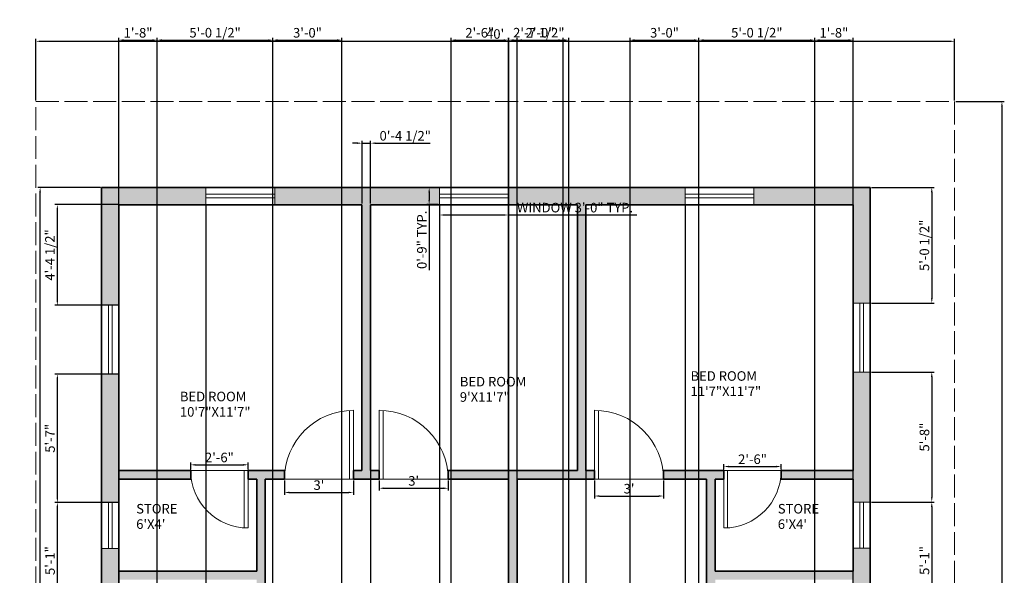
# Model space of a CAD drawing. Units: inches. Extents: x 2871 to 3419, y 1549 to 2228.
# Tile 3 of 3: x 2905 to 3419, y 1938 to 2228. Entities that reach past the tile are written whole.
import ezdxf

# ---------------------------------------------------------------- set-up
doc = ezdxf.new("R2010")
doc.units = ezdxf.units.IN
doc.linetypes.add('ACAD_ISO02W100', pattern=[15, 12, -3])
for name, color, linetype, lineweight in [('A-ANNO-DIMS', 3, 'Continuous', 13), ('A-AREA-IDEN', 3, 'Continuous', 18), ('A-WALL-PATT', 18, 'Continuous', 13), ('C-PROP', 7, 'ACAD_ISO02W100', 18), ('doors', 6, 'Continuous', 18), ('wall', 4, 'Continuous', 35), ('windows', 1, 'Continuous', 18)]:
    doc.layers.add(name, color=color, linetype=linetype, lineweight=lineweight)
doc.styles.get("Standard").update_dxf_attribs({"font": 'arial.ttf', "height": 5})
doc.dimstyles.new('ISO-25', dxfattribs={"dimtxt": 5, "dimasz": 2.5, "dimexe": 1.25, "dimexo": 0.625, "dimtad": 1, "dimlunit": 3, "dimtxsty": 'Standard', "dimcen": 2.5, "dimadec": 0, "dimazin": 0, "dimtfac": 1, "dimtmove": 0, "dimatfit": 3, "dimfxl": 1, "dimarcsym": 0})

# ---------------------------------------------------------------- blocks, each defined once
blk = doc.blocks.new('*D1')
at = {"layer": 'A-ANNO-DIMS', "color": 0, "lineweight": -2, "transparency": 16777216}
for p, q in [((3092.92, 1987.61), (3092.92, 1982.26)), ((3128.92, 1987.61), (3128.92, 1982.26)), ((3095.42, 1983.51), (3126.42, 1983.51))]:
    blk.add_line(p, q, dxfattribs=at)
at = {"layer": 'A-ANNO-DIMS', "color": 0, "transparency": 16777216}
for points in [[(3095.42, 1983.92), (3095.42, 1983.09), (3092.92, 1983.51)], [(3126.42, 1983.92), (3126.42, 1983.09), (3128.92, 1983.51)]]:
    blk.add_solid(points, dxfattribs=at)
at = {"layer": 'Defpoints', "color": 0, "transparency": 16777216}
for p in [(3092.92, 1988.24), (3128.92, 1988.24), (3128.92, 1983.51)]:
    blk.add_point(p, dxfattribs=at)
at = {"layer": 'A-ANNO-DIMS', "color": 0, "transparency": 16777216, "insert": (3110.92, 1986.69), "char_height": 5, "attachment_point": 5}
blk.add_mtext("3'", dxfattribs=at)
blk = doc.blocks.new('*D2')
at = {"layer": 'A-ANNO-DIMS', "color": 0, "lineweight": -2, "transparency": 16777216}
for p, q in [((3043.42, 1987.61), (3043.42, 1980.06)), ((3079.42, 1987.61), (3079.42, 1980.06)), ((3045.92, 1981.31), (3076.92, 1981.31))]:
    blk.add_line(p, q, dxfattribs=at)
at = {"layer": 'A-ANNO-DIMS', "color": 0, "transparency": 16777216}
for points in [[(3045.92, 1981.72), (3045.92, 1980.89), (3043.42, 1981.31)], [(3076.92, 1981.72), (3076.92, 1980.89), (3079.42, 1981.31)]]:
    blk.add_solid(points, dxfattribs=at)
at = {"layer": 'Defpoints', "color": 0, "transparency": 16777216}
for p in [(3043.42, 1988.24), (3079.42, 1988.24), (3079.42, 1981.31)]:
    blk.add_point(p, dxfattribs=at)
at = {"layer": 'A-ANNO-DIMS', "color": 0, "transparency": 16777216, "insert": (3061.42, 1984.49), "char_height": 5, "attachment_point": 5}
blk.add_mtext("3'", dxfattribs=at)
blk = doc.blocks.new('*D3')
at = {"layer": 'A-ANNO-DIMS', "color": 0, "lineweight": -2, "transparency": 16777216}
for p, q in [((2994.42, 1993.36), (2994.42, 1997)), ((2996.92, 1995.75), (3021.92, 1995.75)), ((3024.42, 1993.36), (3024.42, 1997))]:
    blk.add_line(p, q, dxfattribs=at)
at = {"layer": 'A-ANNO-DIMS', "color": 0, "transparency": 16777216}
for points in [[(2996.92, 1996.17), (2996.92, 1995.33), (2994.42, 1995.75)], [(3021.92, 1996.17), (3021.92, 1995.33), (3024.42, 1995.75)]]:
    blk.add_solid(points, dxfattribs=at)
at = {"layer": 'Defpoints', "color": 0, "transparency": 16777216}
for p in [(3024.42, 1995.75), (2994.42, 1992.74), (3024.42, 1992.74)]:
    blk.add_point(p, dxfattribs=at)
at = {"layer": 'A-ANNO-DIMS', "color": 0, "transparency": 16777216, "insert": (3009.42, 1998.93), "char_height": 5, "attachment_point": 5}
blk.add_mtext('2\'-6"', dxfattribs=at)
blk = doc.blocks.new('*D4')
at = {"layer": 'A-ANNO-DIMS', "color": 0, "lineweight": -2, "transparency": 16777216}
for p, q in [((3205.42, 1987.61), (3205.42, 1978.19)), ((3241.42, 1987.61), (3241.42, 1978.19)), ((3207.92, 1979.44), (3238.92, 1979.44))]:
    blk.add_line(p, q, dxfattribs=at)
at = {"layer": 'A-ANNO-DIMS', "color": 0, "transparency": 16777216}
for points in [[(3207.92, 1979.86), (3207.92, 1979.02), (3205.42, 1979.44)], [(3238.92, 1979.86), (3238.92, 1979.02), (3241.42, 1979.44)]]:
    blk.add_solid(points, dxfattribs=at)
at = {"layer": 'Defpoints', "color": 0, "transparency": 16777216}
for p in [(3205.42, 1988.24), (3241.42, 1988.24), (3241.42, 1979.44)]:
    blk.add_point(p, dxfattribs=at)
at = {"layer": 'A-ANNO-DIMS', "color": 0, "transparency": 16777216, "insert": (3223.42, 1982.62), "char_height": 5, "attachment_point": 5}
blk.add_mtext("3'", dxfattribs=at)
blk = doc.blocks.new('*D5')
at = {"layer": 'A-ANNO-DIMS', "color": 0, "lineweight": -2, "transparency": 16777216}
for p, q in [((3272.92, 1993.36), (3272.92, 1996.1)), ((3302.92, 1993.36), (3302.92, 1996.1)), ((3275.42, 1994.85), (3300.42, 1994.85))]:
    blk.add_line(p, q, dxfattribs=at)
at = {"layer": 'A-ANNO-DIMS', "color": 0, "transparency": 16777216}
for points in [[(3275.42, 1995.27), (3275.42, 1994.43), (3272.92, 1994.85)], [(3300.42, 1995.27), (3300.42, 1994.43), (3302.92, 1994.85)]]:
    blk.add_solid(points, dxfattribs=at)
at = {"layer": 'Defpoints', "color": 0, "transparency": 16777216}
for p in [(3272.92, 1992.74), (3302.92, 1994.85), (3302.92, 1992.74)]:
    blk.add_point(p, dxfattribs=at)
at = {"layer": 'A-ANNO-DIMS', "color": 0, "transparency": 16777216, "insert": (3287.92, 1998.03), "char_height": 5, "attachment_point": 5}
blk.add_mtext('2\'-6"', dxfattribs=at)
blk = doc.blocks.new('*D12')
at = {"layer": 'A-ANNO-DIMS', "color": 0, "lineweight": -2, "transparency": 16777216}
for p, q in [((2913.47, 2186.25), (2913.47, 2218.38)), ((2915.97, 2217.13), (3390.97, 2217.13)), ((3393.47, 2186.25), (3393.47, 2218.38))]:
    blk.add_line(p, q, dxfattribs=at)
at = {"layer": 'A-ANNO-DIMS', "color": 0, "transparency": 16777216}
for points in [[(2915.97, 2217.55), (2915.97, 2216.72), (2913.47, 2217.13)], [(3390.97, 2217.55), (3390.97, 2216.72), (3393.47, 2217.13)]]:
    blk.add_solid(points, dxfattribs=at)
at = {"layer": 'Defpoints', "color": 0, "transparency": 16777216}
for p in [(3393.47, 2217.13), (2913.47, 2185.62), (3393.47, 2185.62)]:
    blk.add_point(p, dxfattribs=at)
at = {"layer": 'A-ANNO-DIMS', "color": 0, "transparency": 16777216, "insert": (3153.47, 2220.31), "char_height": 5, "attachment_point": 5}
blk.add_mtext("40'", dxfattribs=at)
blk = doc.blocks.new('*D13')
at = {"layer": 'A-ANNO-DIMS', "color": 0, "lineweight": -2, "transparency": 16777216}
for p, q in [((3394.09, 2185.62), (3419.45, 2185.62)), ((3418.2, 2183.12), (3418.2, 1588.12)), ((3394.09, 1585.62), (3419.45, 1585.62))]:
    blk.add_line(p, q, dxfattribs=at)
at = {"layer": 'A-ANNO-DIMS', "color": 0, "transparency": 16777216}
for points in [[(3417.79, 2183.12), (3418.62, 2183.12), (3418.2, 2185.62)], [(3417.79, 1588.12), (3418.62, 1588.12), (3418.2, 1585.62)]]:
    blk.add_solid(points, dxfattribs=at)
at = {"layer": 'Defpoints', "color": 0, "transparency": 16777216}
for p in [(3393.47, 2185.62), (3393.47, 1585.62), (3418.2, 1585.62)]:
    blk.add_point(p, dxfattribs=at)
at = {"layer": 'A-ANNO-DIMS', "color": 0, "transparency": 16777216, "insert": (3415.03, 1885.62), "char_height": 5, "attachment_point": 5, "rotation": 90}
blk.add_mtext("50'", dxfattribs=at)
blk = doc.blocks.new('WIN-36IN')
for p, q in [((0, 36), (0, 0)), ((9, 36), (0, 36)), ((3.5, 0), (3.5, 36)), ((5.5, 0), (5.5, 36)), ((9, 0), (9, 36)), ((0, 0), (9, 0))]:
    blk.add_line(p, q)
blk = doc.blocks.new('WIN-24IN')
for p, q in [((0, 24), (0, 0)), ((9, 24), (0, 24)), ((3.5, 0), (3.5, 24)), ((5.5, 0), (5.5, 24)), ((9, 0), (9, 24)), ((0, 0), (9, 0))]:
    blk.add_line(p, q)
blk = doc.blocks.new('DOOR-SWING-30IN')
for p, q in [((28, 29.93), (28, 0)), ((30, 30), (30, 0)), ((30, 0), (0, 0))]:
    blk.add_line(p, q)
blk.add_arc((30, 0), 30, 90, 180)
blk = doc.blocks.new('DOOR-SWING-36IN')
for p, q in [((0, 36), (0, 0)), ((2, 35.94), (2, 0)), ((0, 0), (36, 0))]:
    blk.add_line(p, q)
blk.add_arc((0, 0), 36, 0, 90)
blk = doc.blocks.new('*D18')
at = {"layer": 'A-ANNO-DIMS', "color": 0, "lineweight": -2, "transparency": 16777216}
for p, q in [((3124.42, 2131.11), (3124.42, 2125.09)), ((3160.42, 2131.11), (3160.42, 2125.09)), ((3126.92, 2126.34), (3157.92, 2126.34)), ((3160.42, 2126.34), (3227.44, 2126.34))]:
    blk.add_line(p, q, dxfattribs=at)
at = {"layer": 'A-ANNO-DIMS', "color": 0, "transparency": 16777216}
for points in [[(3126.92, 2126.75), (3126.92, 2125.92), (3124.42, 2126.34)], [(3157.92, 2126.75), (3157.92, 2125.92), (3160.42, 2126.34)]]:
    blk.add_solid(points, dxfattribs=at)
at = {"layer": 'Defpoints', "color": 0, "transparency": 16777216}
for p in [(3124.42, 2131.74), (3160.42, 2131.74), (3160.42, 2126.34)]:
    blk.add_point(p, dxfattribs=at)
at = {"layer": 'A-ANNO-DIMS', "color": 0, "transparency": 16777216, "insert": (3195.18, 2129.55), "char_height": 5, "attachment_point": 5}
blk.add_mtext('WINDOW 3\'-0" TYP.', dxfattribs=at)
blk = doc.blocks.new('*D19')
at = {"layer": 'A-ANNO-DIMS', "color": 0, "lineweight": -2, "transparency": 16777216}
for p, q in [((3123.79, 2140.74), (3117.77, 2140.74)), ((3119.02, 2138.24), (3119.02, 2134.24)), ((3123.79, 2131.74), (3117.77, 2131.74)), ((3119.02, 2131.74), (3119.02, 2097.51))]:
    blk.add_line(p, q, dxfattribs=at)
at = {"layer": 'A-ANNO-DIMS', "color": 0, "transparency": 16777216}
for points in [[(3118.6, 2138.24), (3119.43, 2138.24), (3119.02, 2140.74)], [(3118.6, 2134.24), (3119.43, 2134.24), (3119.02, 2131.74)]]:
    blk.add_solid(points, dxfattribs=at)
at = {"layer": 'Defpoints', "color": 0, "transparency": 16777216}
for p in [(3124.42, 2140.74), (3119.02, 2131.74), (3124.42, 2131.74)]:
    blk.add_point(p, dxfattribs=at)
at = {"layer": 'A-ANNO-DIMS', "color": 0, "transparency": 16777216, "insert": (3115.84, 2113.37), "char_height": 5, "attachment_point": 5, "rotation": 90}
blk.add_mtext('0\'-9" TYP.', dxfattribs=at)
blk = doc.blocks.new('*D23')
at = {"layer": 'A-ANNO-DIMS', "color": 0, "lineweight": -2, "transparency": 16777216}
for p, q in [((2947.29, 2140.74), (2914.52, 2140.74)), ((2915.77, 1635.74), (2915.77, 2138.24)), ((2947.29, 1633.24), (2914.52, 1633.24))]:
    blk.add_line(p, q, dxfattribs=at)
at = {"layer": 'A-ANNO-DIMS', "color": 0, "transparency": 16777216}
for points in [[(2915.35, 2138.24), (2916.18, 2138.24), (2915.77, 2140.74)], [(2915.35, 1635.74), (2916.18, 1635.74), (2915.77, 1633.24)]]:
    blk.add_solid(points, dxfattribs=at)
at = {"layer": 'Defpoints', "color": 0, "transparency": 16777216}
for p in [(2915.77, 2140.74), (2947.92, 2140.74), (2947.92, 1633.24)]:
    blk.add_point(p, dxfattribs=at)
at = {"layer": 'A-ANNO-DIMS', "color": 0, "transparency": 16777216, "insert": (2912.56, 1886.99), "char_height": 5, "attachment_point": 5, "rotation": 90}
blk.add_mtext('42\'-3 1/2"', dxfattribs=at)
blk = doc.blocks.new('*D26')
at = {"layer": 'A-ANNO-DIMS', "color": 0, "lineweight": -2, "transparency": 16777216}
for p, q in [((2956.92, 2131.11), (2956.92, 1552.22)), ((3002.42, 2131.11), (3002.42, 1552.22)), ((2959.42, 1553.47), (2999.92, 1553.47))]:
    blk.add_line(p, q, dxfattribs=at)
at = {"layer": 'A-ANNO-DIMS', "color": 0, "transparency": 16777216}
for points in [[(2959.42, 1553.89), (2959.42, 1553.05), (2956.92, 1553.47)], [(2999.92, 1553.89), (2999.92, 1553.05), (3002.42, 1553.47)]]:
    blk.add_solid(points, dxfattribs=at)
at = {"layer": 'Defpoints', "color": 0, "transparency": 16777216}
for p in [(2956.92, 2131.74), (3002.42, 2131.74), (3002.42, 1553.47)]:
    blk.add_point(p, dxfattribs=at)
at = {"layer": 'A-ANNO-DIMS', "color": 0, "transparency": 16777216, "insert": (2979.67, 1556.68), "char_height": 5, "attachment_point": 5}
blk.add_mtext('3\'-9 1/2"', dxfattribs=at)
blk = doc.blocks.new('*D27')
at = {"layer": 'A-ANNO-DIMS', "color": 0, "lineweight": -2, "transparency": 16777216}
for p, q in [((3088.42, 2131.11), (3088.42, 1552.22)), ((3124.42, 2131.11), (3124.42, 1552.22)), ((3090.92, 1553.47), (3121.92, 1553.47))]:
    blk.add_line(p, q, dxfattribs=at)
at = {"layer": 'A-ANNO-DIMS', "color": 0, "transparency": 16777216}
for points in [[(3090.92, 1553.89), (3090.92, 1553.05), (3088.42, 1553.47)], [(3121.92, 1553.89), (3121.92, 1553.05), (3124.42, 1553.47)]]:
    blk.add_solid(points, dxfattribs=at)
at = {"layer": 'Defpoints', "color": 0, "transparency": 16777216}
for p in [(3088.42, 2131.74), (3124.42, 2131.74), (3124.42, 1553.47)]:
    blk.add_point(p, dxfattribs=at)
at = {"layer": 'A-ANNO-DIMS', "color": 0, "transparency": 16777216, "insert": (3106.42, 1556.65), "char_height": 5, "attachment_point": 5}
blk.add_mtext('3\'-0"', dxfattribs=at)
blk = doc.blocks.new('*D28')
at = {"layer": 'A-ANNO-DIMS', "color": 0, "lineweight": -2, "transparency": 16777216}
for p, q in [((3200.92, 2131.11), (3200.92, 1552.22)), ((3252.67, 2131.11), (3252.67, 1552.22)), ((3203.42, 1553.47), (3250.17, 1553.47))]:
    blk.add_line(p, q, dxfattribs=at)
at = {"layer": 'A-ANNO-DIMS', "color": 0, "transparency": 16777216}
for points in [[(3203.42, 1553.89), (3203.42, 1553.05), (3200.92, 1553.47)], [(3250.17, 1553.89), (3250.17, 1553.05), (3252.67, 1553.47)]]:
    blk.add_solid(points, dxfattribs=at)
at = {"layer": 'Defpoints', "color": 0, "transparency": 16777216}
for p in [(3200.92, 2131.74), (3252.67, 2131.74), (3252.67, 1553.47)]:
    blk.add_point(p, dxfattribs=at)
at = {"layer": 'A-ANNO-DIMS', "color": 0, "transparency": 16777216, "insert": (3226.79, 1556.6), "char_height": 5, "attachment_point": 5}
blk.add_mtext('4\'-4"', dxfattribs=at)
blk = doc.blocks.new('*D29')
at = {"layer": 'A-ANNO-DIMS', "color": 0, "lineweight": -2, "transparency": 16777216}
for p, q in [((3130.42, 1871.36), (3130.42, 2219.02)), ((3132.92, 2217.77), (3157.92, 2217.77)), ((3160.42, 1871.36), (3160.42, 2219.02))]:
    blk.add_line(p, q, dxfattribs=at)
at = {"layer": 'A-ANNO-DIMS', "color": 0, "transparency": 16777216}
for points in [[(3132.92, 2218.19), (3132.92, 2217.35), (3130.42, 2217.77)], [(3157.92, 2218.19), (3157.92, 2217.35), (3160.42, 2217.77)]]:
    blk.add_solid(points, dxfattribs=at)
at = {"layer": 'Defpoints', "color": 0, "transparency": 16777216}
for p in [(3160.42, 2217.77), (3130.42, 1870.74), (3160.42, 1870.74)]:
    blk.add_point(p, dxfattribs=at)
at = {"layer": 'A-ANNO-DIMS', "color": 0, "transparency": 16777216, "insert": (3145.42, 2220.95), "char_height": 5, "attachment_point": 5}
blk.add_mtext('2\'-6"', dxfattribs=at)
blk = doc.blocks.new('*D30')
at = {"layer": 'A-ANNO-DIMS', "color": 0, "lineweight": -2, "transparency": 16777216}
for p, q in [((3164.92, 1871.36), (3164.92, 2219.02)), ((3167.42, 2217.77), (3186.42, 2217.77)), ((3188.92, 1871.36), (3188.92, 2219.02))]:
    blk.add_line(p, q, dxfattribs=at)
at = {"layer": 'A-ANNO-DIMS', "color": 0, "transparency": 16777216}
for points in [[(3167.42, 2218.19), (3167.42, 2217.35), (3164.92, 2217.77)], [(3186.42, 2218.19), (3186.42, 2217.35), (3188.92, 2217.77)]]:
    blk.add_solid(points, dxfattribs=at)
at = {"layer": 'Defpoints', "color": 0, "transparency": 16777216}
for p in [(3188.92, 2217.77), (3164.92, 1870.74), (3188.92, 1870.74)]:
    blk.add_point(p, dxfattribs=at)
at = {"layer": 'A-ANNO-DIMS', "color": 0, "transparency": 16777216, "insert": (3176.92, 2220.95), "char_height": 5, "attachment_point": 5}
blk.add_mtext('2\'-0"', dxfattribs=at)
blk = doc.blocks.new('*D34')
at = {"layer": 'A-ANNO-DIMS', "color": 0, "lineweight": -2, "transparency": 16777216}
for p, q in [((3350.04, 2140.74), (3382.82, 2140.74)), ((3381.57, 2138.24), (3381.57, 2082.74)), ((3350.04, 2080.24), (3382.82, 2080.24))]:
    blk.add_line(p, q, dxfattribs=at)
at = {"layer": 'A-ANNO-DIMS', "color": 0, "transparency": 16777216}
for points in [[(3381.15, 2138.24), (3381.98, 2138.24), (3381.57, 2140.74)], [(3381.15, 2082.74), (3381.98, 2082.74), (3381.57, 2080.24)]]:
    blk.add_solid(points, dxfattribs=at)
at = {"layer": 'Defpoints', "color": 0, "transparency": 16777216}
for p in [(3349.42, 2140.74), (3349.42, 2080.24), (3381.57, 2080.24)]:
    blk.add_point(p, dxfattribs=at)
at = {"layer": 'A-ANNO-DIMS', "color": 0, "transparency": 16777216, "insert": (3378.36, 2110.49), "char_height": 5, "attachment_point": 5, "rotation": 90}
blk.add_mtext('5\'-0 1/2"', dxfattribs=at)
blk = doc.blocks.new('*D35')
at = {"layer": 'A-ANNO-DIMS', "color": 0, "lineweight": -2, "transparency": 16777216}
for p, q in [((3350.04, 2044.24), (3382.82, 2044.24)), ((3381.57, 2041.74), (3381.57, 1978.74)), ((3350.04, 1976.24), (3382.82, 1976.24))]:
    blk.add_line(p, q, dxfattribs=at)
at = {"layer": 'A-ANNO-DIMS', "color": 0, "transparency": 16777216}
for points in [[(3381.15, 2041.74), (3381.98, 2041.74), (3381.57, 2044.24)], [(3381.15, 1978.74), (3381.98, 1978.74), (3381.57, 1976.24)]]:
    blk.add_solid(points, dxfattribs=at)
at = {"layer": 'Defpoints', "color": 0, "transparency": 16777216}
for p in [(3349.42, 2044.24), (3349.42, 1976.24), (3381.57, 1976.24)]:
    blk.add_point(p, dxfattribs=at)
at = {"layer": 'A-ANNO-DIMS', "color": 0, "transparency": 16777216, "insert": (3378.39, 2010.24), "char_height": 5, "attachment_point": 5, "rotation": 90}
blk.add_mtext('5\'-8"', dxfattribs=at)
blk = doc.blocks.new('*D36')
at = {"layer": 'A-ANNO-DIMS', "color": 0, "lineweight": -2, "transparency": 16777216}
for p, q in [((3350.04, 1976.24), (3382.82, 1976.24)), ((3381.57, 1973.74), (3381.57, 1917.74)), ((3350.04, 1915.24), (3382.82, 1915.24))]:
    blk.add_line(p, q, dxfattribs=at)
at = {"layer": 'A-ANNO-DIMS', "color": 0, "transparency": 16777216}
for points in [[(3381.15, 1973.74), (3381.98, 1973.74), (3381.57, 1976.24)], [(3381.15, 1917.74), (3381.98, 1917.74), (3381.57, 1915.24)]]:
    blk.add_solid(points, dxfattribs=at)
at = {"layer": 'Defpoints', "color": 0, "transparency": 16777216}
for p in [(3349.42, 1976.24), (3349.42, 1915.24), (3381.57, 1915.24)]:
    blk.add_point(p, dxfattribs=at)
at = {"layer": 'A-ANNO-DIMS', "color": 0, "transparency": 16777216, "insert": (3378.39, 1945.74), "char_height": 5, "attachment_point": 5, "rotation": 90}
blk.add_mtext('5\'-1"', dxfattribs=at)
blk = doc.blocks.new('*D39')
at = {"layer": 'A-ANNO-DIMS', "color": 0, "lineweight": -2, "transparency": 16777216}
for p, q in [((2956.29, 2131.74), (2923.52, 2131.74)), ((2924.77, 2081.65), (2924.77, 2129.24)), ((2956.29, 2079.15), (2923.52, 2079.15))]:
    blk.add_line(p, q, dxfattribs=at)
at = {"layer": 'A-ANNO-DIMS', "color": 0, "transparency": 16777216}
for points in [[(2924.35, 2129.24), (2925.18, 2129.24), (2924.77, 2131.74)], [(2924.35, 2081.65), (2925.18, 2081.65), (2924.77, 2079.15)]]:
    blk.add_solid(points, dxfattribs=at)
at = {"layer": 'Defpoints', "color": 0, "transparency": 16777216}
for p in [(2924.77, 2131.74), (2956.92, 2131.74), (2956.92, 2079.15)]:
    blk.add_point(p, dxfattribs=at)
at = {"layer": 'A-ANNO-DIMS', "color": 0, "transparency": 16777216, "insert": (2921.56, 2105.44), "char_height": 5, "attachment_point": 5, "rotation": 90}
blk.add_mtext('4\'-4 1/2"', dxfattribs=at)
blk = doc.blocks.new('*D40')
at = {"layer": 'A-ANNO-DIMS', "color": 0, "lineweight": -2, "transparency": 16777216}
for p, q in [((2956.29, 2043.15), (2923.52, 2043.15)), ((2924.77, 1978.56), (2924.77, 2040.65)), ((2956.29, 1976.06), (2923.52, 1976.06))]:
    blk.add_line(p, q, dxfattribs=at)
at = {"layer": 'A-ANNO-DIMS', "color": 0, "transparency": 16777216}
for points in [[(2924.35, 2040.65), (2925.18, 2040.65), (2924.77, 2043.15)], [(2924.35, 1978.56), (2925.18, 1978.56), (2924.77, 1976.06)]]:
    blk.add_solid(points, dxfattribs=at)
at = {"layer": 'Defpoints', "color": 0, "transparency": 16777216}
for p in [(2924.77, 2043.15), (2956.92, 2043.15), (2956.92, 1976.06)]:
    blk.add_point(p, dxfattribs=at)
at = {"layer": 'A-ANNO-DIMS', "color": 0, "transparency": 16777216, "insert": (2921.6, 2009.61), "char_height": 5, "attachment_point": 5, "rotation": 90}
blk.add_mtext('5\'-7"', dxfattribs=at)
blk = doc.blocks.new('*D41')
at = {"layer": 'A-ANNO-DIMS', "color": 0, "lineweight": -2, "transparency": 16777216}
for p, q in [((2956.29, 1976.06), (2923.52, 1976.06)), ((2924.77, 1917.79), (2924.77, 1973.56)), ((2956.29, 1915.29), (2923.52, 1915.29))]:
    blk.add_line(p, q, dxfattribs=at)
at = {"layer": 'A-ANNO-DIMS', "color": 0, "transparency": 16777216}
for points in [[(2924.35, 1973.56), (2925.18, 1973.56), (2924.77, 1976.06)], [(2924.35, 1917.79), (2925.18, 1917.79), (2924.77, 1915.29)]]:
    blk.add_solid(points, dxfattribs=at)
at = {"layer": 'Defpoints', "color": 0, "transparency": 16777216}
for p in [(2924.77, 1976.06), (2956.92, 1976.06), (2956.92, 1915.29)]:
    blk.add_point(p, dxfattribs=at)
at = {"layer": 'A-ANNO-DIMS', "color": 0, "transparency": 16777216, "insert": (2921.59, 1945.68), "char_height": 5, "attachment_point": 5, "rotation": 90}
blk.add_mtext('5\'-1"', dxfattribs=at)
blk = doc.blocks.new('*D44')
at = {"layer": 'A-ANNO-DIMS', "color": 0, "lineweight": -2, "transparency": 16777216}
for p, q in [((2956.92, 1683.36), (2956.92, 2219.02)), ((2959.42, 2217.77), (2974.42, 2217.77)), ((2976.92, 1683.36), (2976.92, 2219.02))]:
    blk.add_line(p, q, dxfattribs=at)
at = {"layer": 'A-ANNO-DIMS', "color": 0, "transparency": 16777216}
for points in [[(2959.42, 2218.19), (2959.42, 2217.35), (2956.92, 2217.77)], [(2974.42, 2218.19), (2974.42, 2217.35), (2976.92, 2217.77)]]:
    blk.add_solid(points, dxfattribs=at)
at = {"layer": 'Defpoints', "color": 0, "transparency": 16777216}
for p in [(2976.92, 2217.77), (2956.92, 1682.74), (2976.92, 1682.74)]:
    blk.add_point(p, dxfattribs=at)
at = {"layer": 'A-ANNO-DIMS', "color": 0, "transparency": 16777216, "insert": (2966.92, 2220.95), "char_height": 5, "attachment_point": 5}
blk.add_mtext('1\'-8"', dxfattribs=at)
blk = doc.blocks.new('*D45')
at = {"layer": 'A-ANNO-DIMS', "color": 0, "lineweight": -2, "transparency": 16777216}
for p, q in [((3320.42, 1683.36), (3320.42, 2219.02)), ((3322.92, 2217.77), (3337.92, 2217.77)), ((3340.42, 1683.36), (3340.42, 2219.02))]:
    blk.add_line(p, q, dxfattribs=at)
at = {"layer": 'A-ANNO-DIMS', "color": 0, "transparency": 16777216}
for points in [[(3322.92, 2218.19), (3322.92, 2217.35), (3320.42, 2217.77)], [(3337.92, 2218.19), (3337.92, 2217.35), (3340.42, 2217.77)]]:
    blk.add_solid(points, dxfattribs=at)
at = {"layer": 'Defpoints', "color": 0, "transparency": 16777216}
for p in [(3340.42, 2217.77), (3320.42, 1682.74), (3340.42, 1682.74)]:
    blk.add_point(p, dxfattribs=at)
at = {"layer": 'A-ANNO-DIMS', "color": 0, "transparency": 16777216, "insert": (3330.42, 2220.95), "char_height": 5, "attachment_point": 5}
blk.add_mtext('1\'-8"', dxfattribs=at)
blk = doc.blocks.new('*D46')
at = {"layer": 'A-ANNO-DIMS', "color": 0, "lineweight": -2, "transparency": 16777216}
for p, q in [((3037.42, 1683.36), (3037.42, 2219.02)), ((3039.92, 2217.77), (3070.92, 2217.77)), ((3073.42, 1683.36), (3073.42, 2219.02))]:
    blk.add_line(p, q, dxfattribs=at)
at = {"layer": 'A-ANNO-DIMS', "color": 0, "transparency": 16777216}
for points in [[(3039.92, 2218.19), (3039.92, 2217.35), (3037.42, 2217.77)], [(3070.92, 2218.19), (3070.92, 2217.35), (3073.42, 2217.77)]]:
    blk.add_solid(points, dxfattribs=at)
at = {"layer": 'Defpoints', "color": 0, "transparency": 16777216}
for p in [(3073.42, 2217.77), (3037.42, 1682.74), (3073.42, 1682.74)]:
    blk.add_point(p, dxfattribs=at)
at = {"layer": 'A-ANNO-DIMS', "color": 0, "transparency": 16777216, "insert": (3055.42, 2220.95), "char_height": 5, "attachment_point": 5}
blk.add_mtext('3\'-0"', dxfattribs=at)
blk = doc.blocks.new('*D47')
at = {"layer": 'A-ANNO-DIMS', "color": 0, "lineweight": -2, "transparency": 16777216}
for p, q in [((3223.92, 1683.36), (3223.92, 2219.02)), ((3226.42, 2217.77), (3257.42, 2217.77)), ((3259.92, 1683.36), (3259.92, 2219.02))]:
    blk.add_line(p, q, dxfattribs=at)
at = {"layer": 'A-ANNO-DIMS', "color": 0, "transparency": 16777216}
for points in [[(3226.42, 2218.19), (3226.42, 2217.35), (3223.92, 2217.77)], [(3257.42, 2218.19), (3257.42, 2217.35), (3259.92, 2217.77)]]:
    blk.add_solid(points, dxfattribs=at)
at = {"layer": 'Defpoints', "color": 0, "transparency": 16777216}
for p in [(3259.92, 2217.77), (3223.92, 1682.74), (3259.92, 1682.74)]:
    blk.add_point(p, dxfattribs=at)
at = {"layer": 'A-ANNO-DIMS', "color": 0, "transparency": 16777216, "insert": (3241.92, 2220.95), "char_height": 5, "attachment_point": 5}
blk.add_mtext('3\'-0"', dxfattribs=at)
blk = doc.blocks.new('*D48')
at = {"layer": 'A-ANNO-DIMS', "color": 0, "lineweight": -2, "transparency": 16777216}
for p, q in [((2976.92, 1683.36), (2976.92, 2219.02)), ((2979.42, 2217.77), (3034.92, 2217.77)), ((3037.42, 1683.36), (3037.42, 2219.02))]:
    blk.add_line(p, q, dxfattribs=at)
at = {"layer": 'A-ANNO-DIMS', "color": 0, "transparency": 16777216}
for points in [[(2979.42, 2218.19), (2979.42, 2217.35), (2976.92, 2217.77)], [(3034.92, 2218.19), (3034.92, 2217.35), (3037.42, 2217.77)]]:
    blk.add_solid(points, dxfattribs=at)
at = {"layer": 'Defpoints', "color": 0, "transparency": 16777216}
for p in [(3037.42, 2217.77), (2976.92, 1682.74), (3037.42, 1682.74)]:
    blk.add_point(p, dxfattribs=at)
at = {"layer": 'A-ANNO-DIMS', "color": 0, "transparency": 16777216, "insert": (3007.17, 2220.98), "char_height": 5, "attachment_point": 5}
blk.add_mtext('5\'-0 1/2"', dxfattribs=at)
blk = doc.blocks.new('*D49')
at = {"layer": 'A-ANNO-DIMS', "color": 0, "lineweight": -2, "transparency": 16777216}
for p, q in [((3259.92, 1683.36), (3259.92, 2219.02)), ((3262.42, 2217.77), (3317.92, 2217.77)), ((3320.42, 1683.36), (3320.42, 2219.02))]:
    blk.add_line(p, q, dxfattribs=at)
at = {"layer": 'A-ANNO-DIMS', "color": 0, "transparency": 16777216}
for points in [[(3262.42, 2218.19), (3262.42, 2217.35), (3259.92, 2217.77)], [(3317.92, 2218.19), (3317.92, 2217.35), (3320.42, 2217.77)]]:
    blk.add_solid(points, dxfattribs=at)
at = {"layer": 'Defpoints', "color": 0, "transparency": 16777216}
for p in [(3320.42, 2217.77), (3259.92, 1682.74), (3320.42, 1682.74)]:
    blk.add_point(p, dxfattribs=at)
at = {"layer": 'A-ANNO-DIMS', "color": 0, "transparency": 16777216, "insert": (3290.17, 2220.98), "char_height": 5, "attachment_point": 5}
blk.add_mtext('5\'-0 1/2"', dxfattribs=at)
blk = doc.blocks.new('*D50')
at = {"layer": 'A-ANNO-DIMS', "color": 0, "lineweight": -2, "transparency": 16777216}
for p, q in [((3081.42, 2163.89), (3078.92, 2163.89)), ((3083.92, 2132.36), (3083.92, 2165.14)), ((3083.92, 2163.89), (3088.42, 2163.89)), ((3088.42, 2132.36), (3088.42, 2165.14)), ((3090.92, 2163.89), (3119.61, 2163.89))]:
    blk.add_line(p, q, dxfattribs=at)
at = {"layer": 'A-ANNO-DIMS', "color": 0, "transparency": 16777216}
for points in [[(3081.42, 2164.3), (3081.42, 2163.47), (3083.92, 2163.89)], [(3090.92, 2164.3), (3090.92, 2163.47), (3088.42, 2163.89)]]:
    blk.add_solid(points, dxfattribs=at)
at = {"layer": 'Defpoints', "color": 0, "transparency": 16777216}
for p in [(3088.42, 2163.89), (3083.92, 2131.74), (3088.42, 2131.74)]:
    blk.add_point(p, dxfattribs=at)
at = {"layer": 'A-ANNO-DIMS', "color": 0, "transparency": 16777216, "insert": (3106.51, 2167.1), "char_height": 5, "attachment_point": 5}
blk.add_mtext('0\'-4 1/2"', dxfattribs=at)
blk = doc.blocks.new('*D51')
at = {"layer": 'A-ANNO-DIMS', "color": 0, "lineweight": -2, "transparency": 16777216}
for p, q in [((3160.67, 1683.36), (3160.67, 2219.02)), ((3163.17, 2217.77), (3189.42, 2217.77)), ((3191.92, 1683.36), (3191.92, 2219.02))]:
    blk.add_line(p, q, dxfattribs=at)
at = {"layer": 'A-ANNO-DIMS', "color": 0, "transparency": 16777216}
for points in [[(3163.17, 2218.19), (3163.17, 2217.35), (3160.67, 2217.77)], [(3189.42, 2218.19), (3189.42, 2217.35), (3191.92, 2217.77)]]:
    blk.add_solid(points, dxfattribs=at)
at = {"layer": 'Defpoints', "color": 0, "transparency": 16777216}
for p in [(3191.92, 2217.77), (3160.67, 1682.74), (3191.92, 1682.74)]:
    blk.add_point(p, dxfattribs=at)
at = {"layer": 'A-ANNO-DIMS', "color": 0, "transparency": 16777216, "insert": (3176.29, 2220.98), "char_height": 5, "attachment_point": 5}
blk.add_mtext('2\'-7 1/2"', dxfattribs=at)

msp = doc.modelspace()

# ---------------------------------------------------------------- hatches: boundary and pattern name
at = {"layer": 'A-WALL-PATT'}
h = msp.add_hatch(color=256, dxfattribs=at)
h.dxf.hatch_style = 1
h.paths.add_polyline_path([(2956.918, 2131.735), (3002.418, 2131.735), (3002.418, 2140.735), (2947.918, 2140.735), (2947.918, 2079.154), (2956.918, 2079.154)])
h.paths.add_polyline_path([(3252.668, 2140.735), (3160.418, 2140.735), (3160.418, 2131.735), (3196.418, 2131.735), (3196.418, 1992.735), (3128.918, 1992.735), (3128.918, 1988.235), (3160.418, 1988.235), (3160.418, 1870.735), (3160.418, 1866.235), (3164.918, 1866.235), (3164.918, 1890.235), (3164.918, 1988.235), (3205.418, 1988.235), (3205.418, 1992.735), (3200.918, 1992.735), (3200.918, 2131.735), (3252.668, 2131.735)])
h.paths.add_polyline_path([(3349.418, 2140.735), (3288.668, 2140.735), (3288.668, 2131.735), (3340.418, 2131.735), (3340.418, 2080.235), (3349.418, 2080.235)])
h.paths.add_polyline_path([(3349.418, 2044.235), (3340.418, 2044.235), (3340.418, 1992.735), (3302.918, 1992.735), (3302.918, 1988.235), (3340.418, 1988.235), (3340.418, 1976.235), (3349.418, 1976.235)])
h.paths.add_polyline_path([(3349.418, 1952.235), (3340.418, 1952.235), (3340.418, 1940.235), (3268.418, 1940.235), (3268.418, 1988.235), (3272.918, 1988.235), (3272.918, 1992.735), (3241.418, 1992.735), (3241.418, 1988.235), (3263.918, 1988.235), (3263.918, 1931.235), (3268.418, 1931.235), (3268.418, 1935.735), (3340.418, 1935.735), (3340.418, 1915.235), (3349.418, 1915.235)])
h.paths.add_polyline_path([(3349.418, 1891.235), (3340.418, 1891.235), (3340.418, 1870.735), (3268.418, 1870.735), (3268.418, 1901.235), (3263.918, 1901.235), (3263.918, 1870.735), (3251.918, 1870.735), (3251.918, 1866.235), (3251.918, 1861.735), (3256.418, 1861.735), (3256.418, 1866.235), (3340.418, 1866.235), (3340.418, 1854.235), (3349.418, 1854.235)])
h.paths.add_polyline_path([(3349.418, 1830.235), (3340.418, 1830.235), (3340.418, 1818.235), (3256.418, 1818.235), (3256.418, 1831.735), (3251.918, 1831.735), (3251.918, 1818.235), (3236.918, 1818.235), (3236.918, 1813.735), (3340.418, 1813.735), (3340.418, 1766.452), (3349.418, 1766.452)])
h.paths.add_polyline_path([(3349.418, 1730.452), (3340.418, 1730.452), (3340.418, 1682.735), (3320.418, 1682.735), (3320.418, 1673.735), (3344.918, 1673.735), (3344.918, 1637.735), (3223.918, 1637.735), (3223.918, 1673.735), (3219.418, 1673.735), (3219.418, 1633.235), (3349.418, 1633.235)])
h.paths.add_polyline_path([(3284.418, 1682.735), (3259.918, 1682.735), (3259.918, 1673.735), (3284.418, 1673.735)], flags=17)
h.paths.add_polyline_path([(3223.918, 1682.735), (3219.418, 1682.735), (3219.418, 1673.735), (3223.918, 1673.735)], flags=17)
h.paths.add_polyline_path([(3196.418, 1813.735), (3200.918, 1813.735), (3200.918, 1818.235), (3196.418, 1818.235), (3196.418, 1866.235), (3196.418, 1870.735), (3188.918, 1870.735), (3188.918, 1866.235), (3191.918, 1866.235), (3191.918, 1682.735), (3160.668, 1682.735), (3160.668, 1673.735), (3219.418, 1673.735), (3219.418, 1682.735), (3196.418, 1682.735)])
h.paths.add_polyline_path([(3105.418, 1866.235), (3130.418, 1866.235), (3130.418, 1870.735), (3100.918, 1870.735), (3100.918, 1866.235), (3100.918, 1818.235), (3096.418, 1818.235), (3096.418, 1813.735), (3100.918, 1813.735), (3100.918, 1682.735), (3077.918, 1682.735), (3077.918, 1673.735), (3136.668, 1673.735), (3136.668, 1682.735), (3105.418, 1682.735)])
h.paths.add_polyline_path([(3077.918, 1682.735), (3073.418, 1682.735), (3073.418, 1673.735), (3077.918, 1673.735)], flags=17)
h.paths.add_polyline_path([(3077.918, 1673.735), (3073.418, 1673.735), (3073.418, 1637.735), (2952.418, 1637.735), (2952.418, 1673.735), (2976.918, 1673.735), (2976.918, 1682.735), (2956.918, 1682.735), (2956.918, 1729.593), (2947.918, 1729.593), (2947.918, 1633.235), (3077.918, 1633.235)])
h.paths.add_polyline_path([(3037.418, 1682.735), (3012.918, 1682.735), (3012.918, 1673.735), (3037.418, 1673.735)], flags=17)
h.paths.add_polyline_path([(3060.418, 1818.235), (3045.418, 1818.235), (3045.418, 1831.735), (3040.918, 1831.735), (3040.918, 1818.235), (2956.918, 1818.235), (2956.918, 1830.772), (2947.918, 1830.772), (2947.918, 1765.593), (2956.918, 1765.593), (2956.918, 1813.735), (3060.418, 1813.735)])
h.paths.add_polyline_path([(3045.418, 1870.735), (3033.418, 1870.735), (3033.418, 1901.235), (3028.918, 1901.235), (3028.918, 1870.735), (2956.918, 1870.735), (2956.918, 1891.289), (2947.918, 1891.289), (2947.918, 1854.772), (2956.918, 1854.772), (2956.918, 1866.235), (3040.918, 1866.235), (3040.918, 1861.735), (3045.418, 1861.735), (3045.418, 1866.235)])
h.paths.add_polyline_path([(3033.418, 1988.235), (3043.418, 1988.235), (3043.418, 1992.735), (3024.418, 1992.735), (3024.418, 1988.235), (3028.918, 1988.235), (3028.918, 1940.235), (2956.918, 1940.235), (2956.918, 1952.063), (2947.918, 1952.063), (2947.918, 1915.289), (2956.918, 1915.289), (2956.918, 1935.735), (3028.918, 1935.735), (3028.918, 1931.235), (3033.418, 1931.235)])
h.paths.add_polyline_path([(2956.918, 2043.154), (2947.918, 2043.154), (2947.918, 1976.063), (2956.918, 1976.063), (2956.918, 1988.235), (2994.418, 1988.235), (2994.418, 1992.735), (2956.918, 1992.735)])
h = msp.add_hatch(color=256, dxfattribs=at)
h.dxf.hatch_style = 1
h.paths.add_polyline_path([(3124.418, 2140.735), (3038.418, 2140.735), (3038.418, 2131.735), (3083.918, 2131.735), (3083.918, 1992.735), (3079.418, 1992.735), (3079.418, 1988.235), (3092.918, 1988.235), (3092.918, 1992.735), (3088.418, 1992.735), (3088.418, 2131.735), (3124.418, 2131.735)])

# ---------------------------------------------------------------- linework, layer by layer
at = {"layer": 'C-PROP'}
for p, q in [((2913.468, 2185.622), (3393.468, 2185.622)), ((2913.468, 1585.622), (2913.468, 2185.622)), ((3393.468, 2185.622), (3393.468, 1585.622))]:
    msp.add_line(p, q, dxfattribs=at)
at = {"layer": 'wall'}
for p, q in [((2947.918, 2140.735), (2947.918, 1633.235)), ((3349.418, 2140.735), (2947.918, 2140.735)), ((3349.418, 2140.735), (3349.418, 1633.235)), ((2956.918, 2131.735), (2956.918, 1992.735)), ((3083.918, 2131.735), (2956.918, 2131.735)), ((3083.918, 2131.735), (3083.918, 1992.735)), ((3088.418, 2131.735), (3088.418, 1992.735)), ((3196.418, 2131.735), (3088.418, 2131.735)), ((3196.418, 2131.735), (3196.418, 1992.735)), ((3340.418, 2131.735), (3200.918, 2131.735)), ((3200.918, 2131.735), (3200.918, 1992.735)), ((3340.418, 2131.735), (3340.418, 1992.735)), ((2994.418, 1992.735), (2956.918, 1992.735)), ((2994.418, 1988.235), (2994.418, 1992.735)), ((3024.418, 1988.235), (3024.418, 1992.735)), ((3043.418, 1992.735), (3024.418, 1992.735)), ((3043.418, 1992.735), (3043.418, 1988.235)), ((3083.918, 1992.735), (3079.418, 1992.735)), ((3079.418, 1992.735), (3079.418, 1988.235)), ((3083.918, 1992.735), (3083.918, 1992.735)), ((3092.918, 1992.735), (3088.418, 1992.735)), ((3092.918, 1992.735), (3092.918, 1988.235)), ((3196.418, 1992.735), (3128.918, 1992.735)), ((3128.918, 1992.735), (3128.918, 1988.235)), ((3205.418, 1992.735), (3200.918, 1992.735)), ((3205.418, 1992.735), (3205.418, 1988.235)), ((3241.418, 1992.735), (3241.418, 1988.235)), ((3272.918, 1992.735), (3241.418, 1992.735)), ((3272.918, 1988.235), (3272.918, 1992.735)), ((3340.418, 1992.735), (3302.918, 1992.735)), ((3302.918, 1988.235), (3302.918, 1992.735)), ((2956.918, 1988.235), (2956.918, 1940.235)), ((2994.418, 1988.235), (2956.918, 1988.235)), ((3028.918, 1988.235), (3024.418, 1988.235)), ((3028.918, 1988.235), (3028.918, 1940.235)), ((3033.418, 1988.235), (3033.418, 1931.235)), ((3043.418, 1988.235), (3033.418, 1988.235)), ((3092.918, 1988.235), (3079.418, 1988.235)), ((3160.418, 1988.235), (3128.918, 1988.235)), ((3160.418, 1988.235), (3160.418, 1870.735)), ((3164.918, 1988.235), (3164.918, 1870.735)), ((3205.418, 1988.235), (3164.918, 1988.235)), ((3263.918, 1988.235), (3241.418, 1988.235)), ((3263.918, 1988.235), (3263.918, 1931.235)), ((3268.418, 1988.235), (3268.418, 1940.235)), ((3272.918, 1988.235), (3268.418, 1988.235)), ((3340.418, 1988.235), (3302.918, 1988.235)), ((3340.418, 1988.235), (3340.418, 1940.235)), ((3028.918, 1940.235), (2956.918, 1940.235)), ((3340.418, 1940.235), (3268.418, 1940.235))]:
    msp.add_line(p, q, dxfattribs=at)

# ---------------------------------------------------------------- block references
at = {"layer": 'doors', "extrusion": (0, 0, -1), "zscale": -1}
msp.add_blockref('DOOR-SWING-36IN', (-3079.419, 1988.235), dxfattribs=at)
at = {"layer": 'doors'}
for p in [(3092.918, 1988.235), (3205.418, 1988.235)]:
    msp.add_blockref('DOOR-SWING-36IN', p, dxfattribs=at)
at = {"layer": 'doors', "extrusion": (0, 0, -1), "zscale": -1, "rotation": 180}
msp.add_blockref('DOOR-SWING-30IN', (-2994.418, 1992.735), dxfattribs=at)
at = {"layer": 'doors', "rotation": 180}
msp.add_blockref('DOOR-SWING-30IN', (3302.919, 1992.735), dxfattribs=at)
at = {"layer": 'windows'}
for p, rotation in [((3002.418, 2140.735), 269.999999999999), ((3124.418, 2140.735), 269.9999999999983), ((3252.668, 2140.735), 269.999999999999), ((2956.919, 2079.154), 180)]:
    msp.add_blockref('WIN-36IN', p, dxfattribs=dict(at, rotation=rotation))
for name, p in [('WIN-36IN', (3340.418, 2044.235)), ('WIN-24IN', (2947.918, 1952.063)), ('WIN-24IN', (3340.418, 1952.235))]:
    msp.add_blockref(name, p, dxfattribs=at)

# ---------------------------------------------------------------- texts
at = {"layer": 'A-AREA-IDEN'}
for s, p in [('BED ROOM', (3255.536, 2039.679)), ('BED ROOM', (3135.028, 2036.718)), ('11\'7"X11\'7"', (3255.536, 2031.647)), ('BED ROOM', (2988.795, 2028.955)), ('9\'X11\'7"', (3135.028, 2028.686)), ('10\'7"X11\'7"', (2988.795, 2020.923)), ('STORE', (2965.967, 1970.285)), ('STORE', (3301.119, 1970.285)), ("6'X4'", (2965.967, 1962.253)), ("6'X4'", (3301.119, 1962.253))]:
    msp.add_text(s, height=5, dxfattribs=at).set_placement(p)

# ---------------------------------------------------------------- dimensions: what is measured, and where the dimension line sits
at = {"layer": 'A-ANNO-DIMS'}
for base, p1, p2, override, picture, middle in [((3037.418, 2217.772), (2976.918, 1682.735), (3037.418, 1682.735), {"dimdec": 1, "dimlfac": 1, "dimrnd": 0, "dimzin": 1, "dimdsep": 46, "dimlunit": 4, "dimfrac": 2}, '*D48', (3007.168, 2220.982)), ((3191.918308, 2217.771512), (3160.668308, 1682.735115), (3191.918308, 1682.735115), {"dimdec": 1, "dimlfac": 1, "dimrnd": 0, "dimzin": 1, "dimdsep": 46, "dimlunit": 4, "dimfrac": 2}, '*D51', (3176.293308, 2220.98177803)), ((3320.418, 2217.772), (3259.918, 1682.735), (3320.418, 1682.735), {"dimdec": 1, "dimlfac": 1, "dimrnd": 0, "dimzin": 1, "dimdsep": 46, "dimlunit": 4, "dimfrac": 2}, '*D49', (3290.168, 2220.982)), ((3393.468, 2217.133), (2913.468, 2185.622), (3393.468, 2185.622), {"dimclrd": 0, "dimclre": 0, "dimclrt": 0}, '*D12', (3153.468, 2220.311)), ((2976.918, 2217.772), (2956.918, 1682.735), (2976.918, 1682.735), {"dimdec": 1, "dimlfac": 1, "dimrnd": 0, "dimzin": 1, "dimdsep": 46, "dimlunit": 4, "dimfrac": 2}, '*D44', (2966.918, 2220.949)), ((3073.418, 2217.772), (3037.418, 1682.735), (3073.418, 1682.735), {"dimdec": 1, "dimlfac": 1, "dimrnd": 0, "dimzin": 1, "dimdsep": 46, "dimlunit": 4, "dimfrac": 2}, '*D46', (3055.418, 2220.951)), ((3160.418, 2217.772), (3130.418, 1870.735), (3160.418, 1870.735), {"dimdec": 1, "dimlfac": 1, "dimrnd": 0, "dimzin": 1, "dimdsep": 46, "dimlunit": 4, "dimfrac": 2}, '*D29', (3145.418, 2220.949)), ((3188.918, 2217.772), (3164.918, 1870.735), (3188.918, 1870.735), {"dimdec": 1, "dimlfac": 1, "dimrnd": 0, "dimzin": 1, "dimdsep": 46, "dimlunit": 4, "dimfrac": 2}, '*D30', (3176.918, 2220.949)), ((3259.918, 2217.772), (3223.918, 1682.735), (3259.918, 1682.735), {"dimdec": 1, "dimlfac": 1, "dimrnd": 0, "dimzin": 1, "dimdsep": 46, "dimlunit": 4, "dimfrac": 2}, '*D47', (3241.918, 2220.951)), ((3340.418, 2217.772), (3320.418, 1682.735), (3340.418, 1682.735), {"dimdec": 1, "dimlfac": 1, "dimrnd": 0, "dimzin": 1, "dimdsep": 46, "dimlunit": 4, "dimfrac": 2}, '*D45', (3330.418, 2220.949)), ((3088.418, 2163.885), (3083.918, 2131.735), (3088.418, 2131.735), {"dimdec": 1, "dimlfac": 1, "dimrnd": 0, "dimzin": 1, "dimdsep": 46, "dimlunit": 4, "dimfrac": 2}, '*D50', (3106.514, 2167.095)), ((3002.418, 1553.472), (2956.918, 2131.735), (3002.418, 2131.735), {"dimdec": 1, "dimlfac": 1, "dimrnd": 0, "dimzin": 1, "dimdsep": 46, "dimlunit": 4, "dimfrac": 2}, '*D26', (2979.668, 1556.683)), ((3124.418, 1553.472), (3088.418, 2131.735), (3124.418, 2131.735), {"dimdec": 1, "dimlfac": 1, "dimrnd": 0, "dimzin": 1, "dimdsep": 46, "dimlunit": 4, "dimfrac": 2}, '*D27', (3106.418, 1556.651)), ((3252.668308, 1553.471512), (3200.918308, 2131.735115), (3252.668308, 2131.735115), {"dimdec": 1, "dimlfac": 1, "dimrnd": 0, "dimzin": 1, "dimdsep": 46, "dimlunit": 4, "dimfrac": 2}, '*D28', (3226.793308, 1556.596512)), ((3024.418, 1995.749), (2994.418, 1992.735), (3024.418, 1992.735), {"dimclrd": 0, "dimclre": 0, "dimclrt": 0}, '*D3', (3009.418, 1998.927)), ((3302.918, 1994.849), (3272.918, 1992.735), (3302.918, 1992.735), {"dimclrd": 0, "dimclre": 0, "dimclrt": 0}, '*D5', (3287.918, 1998.026)), ((3079.418, 1981.308), (3043.418, 1988.235), (3079.418, 1988.235), {"dimclrd": 0, "dimclre": 0, "dimclrt": 0}, '*D2', (3061.418, 1984.487)), ((3128.918, 1983.505), (3092.918, 1988.235), (3128.918, 1988.235), {"dimclrd": 0, "dimclre": 0, "dimclrt": 0}, '*D1', (3110.918, 1986.685)), ((3241.418, 1979.441), (3205.418, 1988.235), (3241.418, 1988.235), {"dimclrd": 0, "dimclre": 0, "dimclrt": 0}, '*D4', (3223.418, 1982.62))]:
    dim = msp.add_linear_dim(base=base, p1=p1, p2=p2, dimstyle='ISO-25', override=override, dxfattribs=at)
    dim.commit()
    dim.dimension.update_dxf_attribs({"geometry": picture, "text_midpoint": middle})
for base, p1, p2, angle, override, picture, middle in [((3418.204, 1585.622), (3393.468, 2185.622), (3393.468, 1585.622), 90, {"dimclrd": 0, "dimclre": 0, "dimclrt": 0}, '*D13', (3415.026, 1885.622)), ((2915.768, 2140.735), (2947.918, 1633.235), (2947.918, 2140.735), 90, {"dimdec": 1, "dimlfac": 1, "dimrnd": 0, "dimzin": 1, "dimdsep": 46, "dimlunit": 4, "dimfrac": 2}, '*D23', (2912.556, 1886.985)), ((3381.568, 2080.235), (3349.418, 2140.735), (3349.418, 2080.235), 270, {"dimdec": 1, "dimlfac": 1, "dimrnd": 0, "dimzin": 1, "dimdsep": 46, "dimlunit": 4, "dimfrac": 2}, '*D34', (3378.358, 2110.485)), ((2924.768, 2131.735), (2956.918, 2079.154), (2956.918, 2131.735), 90, {"dimdec": 1, "dimlfac": 1, "dimrnd": 0, "dimzin": 1, "dimdsep": 46, "dimlunit": 4, "dimfrac": 2}, '*D39', (2921.558, 2105.444)), ((2924.768, 2043.154), (2956.918, 1976.063), (2956.918, 2043.154), 90, {"dimdec": 1, "dimlfac": 1, "dimrnd": 0, "dimzin": 1, "dimdsep": 46, "dimlunit": 4, "dimfrac": 2}, '*D40', (2921.601, 2009.608)), ((3381.568, 1976.235), (3349.418, 2044.235), (3349.418, 1976.235), 270, {"dimdec": 1, "dimlfac": 1, "dimrnd": 0, "dimzin": 1, "dimdsep": 46, "dimlunit": 4, "dimfrac": 2}, '*D35', (3378.39, 2010.235)), ((2924.768, 1976.063), (2956.918, 1915.289), (2956.918, 1976.063), 90, {"dimdec": 1, "dimlfac": 1, "dimrnd": 0, "dimzin": 1, "dimdsep": 46, "dimlunit": 4, "dimfrac": 2}, '*D41', (2921.59, 1945.676)), ((3381.568, 1915.235), (3349.418, 1976.235), (3349.418, 1915.235), 270, {"dimdec": 1, "dimlfac": 1, "dimrnd": 0, "dimzin": 1, "dimdsep": 46, "dimlunit": 4, "dimfrac": 2}, '*D36', (3378.39, 1945.735))]:
    dim = msp.add_linear_dim(base=base, p1=p1, p2=p2, angle=angle, dimstyle='ISO-25', override=override, dxfattribs=at)
    dim.commit()
    dim.dimension.update_dxf_attribs({"geometry": picture, "text_midpoint": middle})
dim = msp.add_linear_dim(base=(3119.018, 2131.735), p1=(3124.418, 2140.735), p2=(3124.418, 2131.735), angle=270, text='<> TYP.', dimstyle='ISO-25', override={"dimdec": 1, "dimlfac": 1, "dimrnd": 0, "dimzin": 1, "dimdsep": 46, "dimlunit": 4, "dimfrac": 2}, dxfattribs=at)
dim.commit()
dim.dimension.update_dxf_attribs({"geometry": '*D19', "text_midpoint": (3115.84, 2113.371)})
dim = msp.add_linear_dim(base=(3160.418, 2126.335), p1=(3124.418, 2131.735), p2=(3160.418, 2131.735), text='WINDOW <> TYP.', dimstyle='ISO-25', override={"dimdec": 1, "dimlfac": 1, "dimrnd": 0, "dimzin": 1, "dimdsep": 46, "dimlunit": 4, "dimfrac": 2}, dxfattribs=at)
dim.commit()
dim.dimension.update_dxf_attribs({"geometry": '*D18', "text_midpoint": (3195.179, 2129.549)})

doc.saveas('drawing.dxf')
